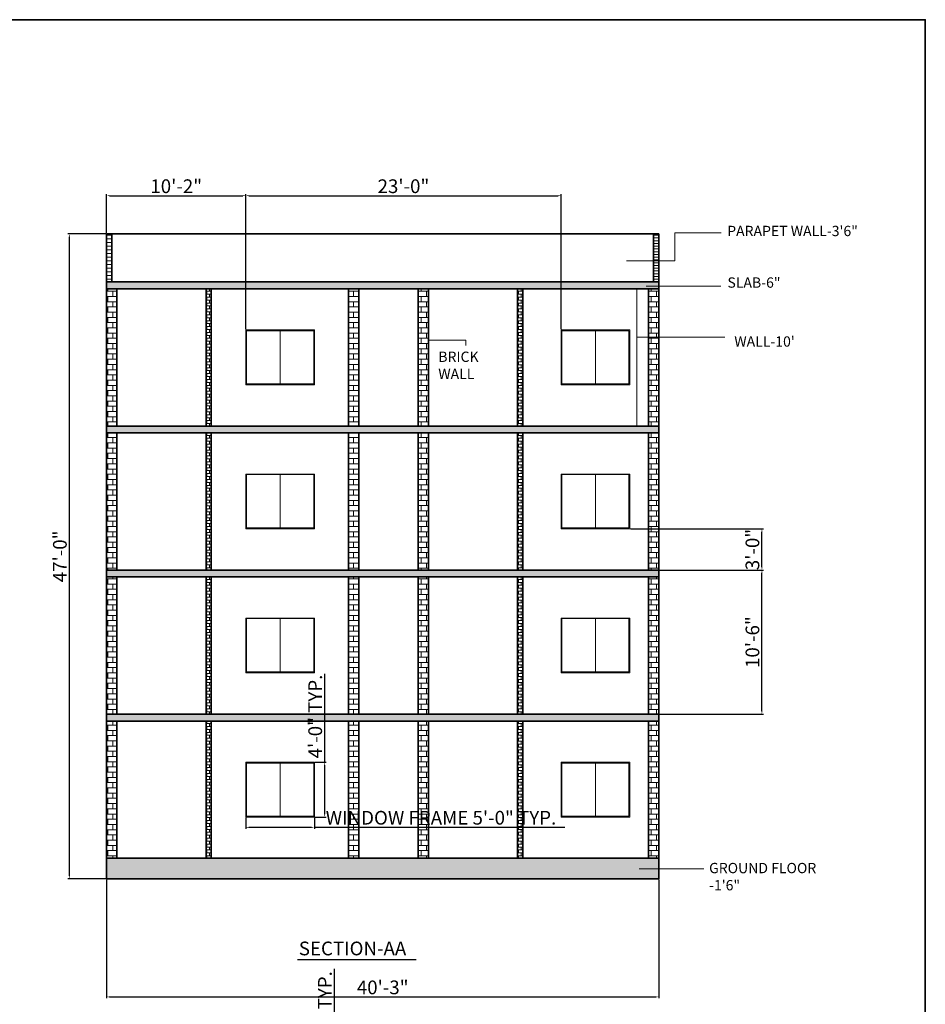
# Model space of a CAD drawing. Units: inches. Extents: x 1266 to 2869, y -408 to 3241.
# Tile 11 of 11: x 2076 to 2869, y 2380 to 3241. Entities that reach past the tile are written whole.
import ezdxf

# ---------------------------------------------------------------- set-up
doc = ezdxf.new("R2010")
doc.units = ezdxf.units.IN
for name, color, linetype, lineweight in [('A-ANNO-DIMS', 2, 'Continuous', 18), ('A-ANNO-TEXT', 7, 'Continuous', 18), ('A-ANNO-TITL', 7, 'Continuous', 25), ('A-ANNO-TTLB', 7, 'Continuous', 35), ('A-GLAZ', 4, 'Continuous', 18), ('A-SECT', 7, 'Continuous', 35), ('A-SECT-PATT', 252, 'Continuous', 13), ('A-SECT-PATT-CONC', 8, 'Continuous', 13), ('A-SECT-PATT-MASN', 8, 'Continuous', 13)]:
    doc.layers.add(name, color=color, linetype=linetype, lineweight=lineweight)
doc.styles.get("Standard").update_dxf_attribs({"font": 'arial.ttf'})
doc.dimstyles.new('ISO-25', dxfattribs={"dimtxt": 12, "dimasz": 2.5, "dimexe": 1.25, "dimexo": 0.625, "dimtad": 1, "dimdec": 0, "dimlunit": 3, "dimtxsty": 'Standard', "dimcen": 2.5, "dimadec": 0, "dimazin": 0, "dimtfac": 1, "dimtdec": 0, "dimtmove": 0, "dimatfit": 3, "dimfxl": 1, "dimarcsym": 0})

# ---------------------------------------------------------------- blocks, each defined once
blk = doc.blocks.new('WIN-SECTION-FRAME-60X48')
for p, q in [((0, 48), (0, 0)), ((0, 48), (60, 48)), ((60, 48), (60, 0)), ((0, 0), (60, 0))]:
    blk.add_line(p, q)
blk = doc.blocks.new('*D39')
at = {"layer": 'A-ANNO-DIMS', "color": 0, "lineweight": -2, "transparency": 16777216}
for p, q in [((2351.77, 2267.74), (2351.77, 2411.2)), ((2339.28, 2267.74), (2353.02, 2267.74)), ((2351.77, 2182.78), (2351.77, 2265.24)), ((2339.28, 2180.28), (2353.02, 2180.28))]:
    blk.add_line(p, q, dxfattribs=at)
at = {"layer": 'A-ANNO-DIMS', "color": 0, "transparency": 16777216}
for points in [[(2351.36, 2265.24), (2352.19, 2265.24), (2351.77, 2267.74)], [(2351.36, 2182.78), (2352.19, 2182.78), (2351.77, 2180.28)]]:
    blk.add_solid(points, dxfattribs=at)
at = {"layer": 'Defpoints', "color": 0, "transparency": 16777216}
for p in [(2338.65, 2267.74), (2351.77, 2267.74), (2338.65, 2180.28)]:
    blk.add_point(p, dxfattribs=at)
at = {"layer": 'A-ANNO-DIMS', "color": 0, "transparency": 16777216, "insert": (2344.94, 2340.72), "char_height": 12, "attachment_point": 5, "rotation": 90}
blk.add_mtext('BED 7\'-3 1/2" TYP.', dxfattribs=at)
blk = doc.blocks.new('*D51')
at = {"layer": 'A-ANNO-DIMS', "color": 0, "lineweight": -2, "transparency": 16777216}
for p, q in [((2274.21, 2543.33), (2274.21, 2533.71)), ((2334.21, 2543.33), (2334.21, 2533.71)), ((2276.71, 2534.96), (2331.71, 2534.96)), ((2334.21, 2534.96), (2553.14, 2534.96))]:
    blk.add_line(p, q, dxfattribs=at)
at = {"layer": 'A-ANNO-DIMS', "color": 0, "transparency": 16777216}
for points in [[(2276.71, 2535.38), (2276.71, 2534.54), (2274.21, 2534.96)], [(2331.71, 2535.38), (2331.71, 2534.54), (2334.21, 2534.96)]]:
    blk.add_solid(points, dxfattribs=at)
at = {"layer": 'Defpoints', "color": 0, "transparency": 16777216}
for p in [(2274.21, 2543.96), (2334.21, 2543.96), (2334.21, 2534.96)]:
    blk.add_point(p, dxfattribs=at)
at = {"layer": 'A-ANNO-DIMS', "color": 0, "transparency": 16777216, "insert": (2444.92, 2541.79), "char_height": 12, "attachment_point": 5}
blk.add_mtext('WINDOW FRAME 5\'-0" TYP.', dxfattribs=at)
blk = doc.blocks.new('*D52')
at = {"layer": 'A-ANNO-DIMS', "color": 0, "lineweight": -2, "transparency": 16777216}
for p, q in [((2343.21, 2591.96), (2343.21, 2669.34)), ((2334.83, 2591.96), (2344.46, 2591.96)), ((2343.21, 2546.46), (2343.21, 2589.46)), ((2334.83, 2543.96), (2344.46, 2543.96))]:
    blk.add_line(p, q, dxfattribs=at)
at = {"layer": 'A-ANNO-DIMS', "color": 0, "transparency": 16777216}
for points in [[(2342.79, 2589.46), (2343.63, 2589.46), (2343.21, 2591.96)], [(2342.79, 2546.46), (2343.63, 2546.46), (2343.21, 2543.96)]]:
    blk.add_solid(points, dxfattribs=at)
at = {"layer": 'Defpoints', "color": 0, "transparency": 16777216}
for p in [(2334.21, 2591.96), (2343.21, 2591.96), (2334.21, 2543.96)]:
    blk.add_point(p, dxfattribs=at)
at = {"layer": 'A-ANNO-DIMS', "color": 0, "transparency": 16777216, "insert": (2336.46, 2631.9), "char_height": 12, "attachment_point": 5, "rotation": 90}
blk.add_mtext('4\'-0" TYP.', dxfattribs=at)
blk = doc.blocks.new('*D96')
at = {"layer": 'A-ANNO-DIMS', "color": 0, "lineweight": -2, "transparency": 16777216}
for p, q in [((2152.45, 2489.33), (2152.45, 2385.4)), ((2635.45, 2489.33), (2635.45, 2385.4)), ((2154.95, 2386.65), (2632.95, 2386.65))]:
    blk.add_line(p, q, dxfattribs=at)
at = {"layer": 'A-ANNO-DIMS', "color": 0, "transparency": 16777216}
for points in [[(2154.95, 2387.07), (2154.95, 2386.23), (2152.45, 2386.65)], [(2632.95, 2387.07), (2632.95, 2386.23), (2635.45, 2386.65)]]:
    blk.add_solid(points, dxfattribs=at)
at = {"layer": 'Defpoints', "color": 0, "transparency": 16777216}
for p in [(2152.45, 2489.96), (2635.45, 2489.96), (2635.45, 2386.65)]:
    blk.add_point(p, dxfattribs=at)
at = {"layer": 'A-ANNO-DIMS', "color": 0, "transparency": 16777216, "insert": (2393.95, 2393.41), "char_height": 12, "attachment_point": 5}
blk.add_mtext('40\'-3"', dxfattribs=at)
blk = doc.blocks.new('*D97')
at = {"layer": 'A-ANNO-DIMS', "color": 0, "lineweight": -2, "transparency": 16777216}
for p, q in [((2151.83, 3053.96), (2118.6, 3053.96)), ((2119.85, 2492.46), (2119.85, 3051.46)), ((2151.83, 2489.96), (2118.6, 2489.96))]:
    blk.add_line(p, q, dxfattribs=at)
at = {"layer": 'A-ANNO-DIMS', "color": 0, "transparency": 16777216}
for points in [[(2119.43, 3051.46), (2120.27, 3051.46), (2119.85, 3053.96)], [(2119.43, 2492.46), (2120.27, 2492.46), (2119.85, 2489.96)]]:
    blk.add_solid(points, dxfattribs=at)
at = {"layer": 'Defpoints', "color": 0, "transparency": 16777216}
for p in [(2119.85, 3053.96), (2152.45, 3053.96), (2152.45, 2489.96)]:
    blk.add_point(p, dxfattribs=at)
at = {"layer": 'A-ANNO-DIMS', "color": 0, "transparency": 16777216, "insert": (2113.1, 2771.96), "char_height": 12, "attachment_point": 5, "rotation": 90}
blk.add_mtext('47\'-0"', dxfattribs=at)
blk = doc.blocks.new('*D98')
at = {"layer": 'A-ANNO-DIMS', "color": 0, "lineweight": -2, "transparency": 16777216}
for p, q in [((2636.08, 2759.96), (2726.95, 2759.96)), ((2725.7, 2636.46), (2725.7, 2757.46)), ((2636.08, 2633.96), (2726.95, 2633.96))]:
    blk.add_line(p, q, dxfattribs=at)
at = {"layer": 'A-ANNO-DIMS', "color": 0, "transparency": 16777216}
for points in [[(2725.28, 2757.46), (2726.12, 2757.46), (2725.7, 2759.96)], [(2725.28, 2636.46), (2726.12, 2636.46), (2725.7, 2633.96)]]:
    blk.add_solid(points, dxfattribs=at)
at = {"layer": 'Defpoints', "color": 0, "transparency": 16777216}
for p in [(2635.45, 2759.96), (2725.7, 2759.96), (2635.45, 2633.96)]:
    blk.add_point(p, dxfattribs=at)
at = {"layer": 'A-ANNO-DIMS', "color": 0, "transparency": 16777216, "insert": (2718.95, 2696.96), "char_height": 12, "attachment_point": 5, "rotation": 90}
blk.add_mtext('10\'-6"', dxfattribs=at)
blk = doc.blocks.new('*D99')
at = {"layer": 'A-ANNO-DIMS', "color": 0, "lineweight": -2, "transparency": 16777216}
for p, q in [((2152.45, 3054.58), (2152.45, 3088.64)), ((2154.95, 3087.39), (2271.71, 3087.39)), ((2274.21, 2970.58), (2274.21, 3088.64))]:
    blk.add_line(p, q, dxfattribs=at)
at = {"layer": 'A-ANNO-DIMS', "color": 0, "transparency": 16777216}
for points in [[(2154.95, 3087.8), (2154.95, 3086.97), (2152.45, 3087.39)], [(2271.71, 3087.8), (2271.71, 3086.97), (2274.21, 3087.39)]]:
    blk.add_solid(points, dxfattribs=at)
at = {"layer": 'Defpoints', "color": 0, "transparency": 16777216}
for p in [(2274.21, 3087.39), (2152.45, 3053.96), (2274.21, 2969.96)]:
    blk.add_point(p, dxfattribs=at)
at = {"layer": 'A-ANNO-DIMS', "color": 0, "transparency": 16777216, "insert": (2213.33, 3094.14), "char_height": 12, "attachment_point": 5}
blk.add_mtext('10\'-2"', dxfattribs=at)
blk = doc.blocks.new('*D100')
at = {"layer": 'A-ANNO-DIMS', "color": 0, "lineweight": -2, "transparency": 16777216}
for p, q in [((2274.21, 2970.58), (2274.21, 3088.64)), ((2276.71, 3087.39), (2547.51, 3087.39)), ((2550.01, 2970.58), (2550.01, 3088.64))]:
    blk.add_line(p, q, dxfattribs=at)
at = {"layer": 'A-ANNO-DIMS', "color": 0, "transparency": 16777216}
for points in [[(2276.71, 3087.8), (2276.71, 3086.97), (2274.21, 3087.39)], [(2547.51, 3087.8), (2547.51, 3086.97), (2550.01, 3087.39)]]:
    blk.add_solid(points, dxfattribs=at)
at = {"layer": 'Defpoints', "color": 0, "transparency": 16777216}
for p in [(2550.01, 3087.39), (2274.21, 2969.96), (2550.01, 2969.96)]:
    blk.add_point(p, dxfattribs=at)
at = {"layer": 'A-ANNO-DIMS', "color": 0, "transparency": 16777216, "insert": (2412.11, 3094.14), "char_height": 12, "attachment_point": 5}
blk.add_mtext('23\'-0"', dxfattribs=at)
blk = doc.blocks.new('*D101')
at = {"layer": 'A-ANNO-DIMS', "color": 0, "lineweight": -2, "transparency": 16777216}
for p, q in [((2610.64, 2795.96), (2726.95, 2795.96)), ((2725.7, 2762.46), (2725.7, 2793.46)), ((2636.08, 2759.96), (2726.95, 2759.96))]:
    blk.add_line(p, q, dxfattribs=at)
at = {"layer": 'A-ANNO-DIMS', "color": 0, "transparency": 16777216}
for points in [[(2725.28, 2793.46), (2726.12, 2793.46), (2725.7, 2795.96)], [(2725.28, 2762.46), (2726.12, 2762.46), (2725.7, 2759.96)]]:
    blk.add_solid(points, dxfattribs=at)
at = {"layer": 'Defpoints', "color": 0, "transparency": 16777216}
for p in [(2610.01, 2795.96), (2725.7, 2795.96), (2635.45, 2759.96)]:
    blk.add_point(p, dxfattribs=at)
at = {"layer": 'A-ANNO-DIMS', "color": 0, "transparency": 16777216, "insert": (2718.94, 2777.96), "char_height": 12, "attachment_point": 5, "rotation": 90}
blk.add_mtext('3\'-0"', dxfattribs=at)

msp = doc.modelspace()

# ---------------------------------------------------------------- hatches: boundary and pattern name
at = {"layer": 'A-SECT-PATT', "transparency": 33554536}
h = msp.add_hatch(color=256, dxfattribs=at)
h.dxf.hatch_style = 1
h.paths.add_polyline_path([(2635.45, 3011.96), (2152.45, 3011.96), (2152.45, 3005.96), (2635.45, 3005.96)])
h.paths.add_polyline_path([(2635.45, 2885.96), (2152.45, 2885.96), (2152.45, 2879.96), (2635.45, 2879.96)])
h.paths.add_polyline_path([(2635.45, 2759.96), (2152.45, 2759.96), (2152.45, 2753.96), (2635.45, 2753.96)])
h.paths.add_polyline_path([(2635.45, 2633.96), (2152.45, 2633.96), (2152.45, 2627.96), (2635.45, 2627.96)])
at = {"layer": 'A-SECT-PATT-CONC'}
h = msp.add_hatch(dxfattribs=at)
h.set_pattern_fill('AR-CONC', color=256, scale=0.107, style=0)
h.paths.add_polyline_path([(2152.45, 2489.96), (2635.45, 2489.96), (2635.45, 2507.96), (2152.45, 2507.96)])
at = {"layer": 'A-SECT-PATT-MASN'}
h = msp.add_hatch(dxfattribs=at)
h.set_pattern_fill('LINE', color=256, scale=1.007874, style=0)
h.paths.add_polyline_path([(2152.45, 3011.96), (2157.08, 3011.96), (2157.08, 3053.96), (2152.45, 3053.96)])
h = msp.add_hatch(dxfattribs=at)
h.set_pattern_fill('LINE', color=256, scale=0.7559055, style=0)
h.paths.add_polyline_path([(2630.96, 3011.96), (2635.45, 3011.96), (2635.45, 3053.96), (2630.96, 3053.96)])
h = msp.add_hatch(dxfattribs=at)
h.set_pattern_fill('BRICK', color=256, scale=0.72, style=0)
h.paths.add_polyline_path([(2152.45, 2885.96), (2161.45, 2885.96), (2161.45, 3005.96), (2152.45, 3005.96)])
h = msp.add_hatch(dxfattribs=at)
h.set_pattern_fill('BRICK', color=256, scale=0.405, style=0)
h.paths.add_polyline_path([(2239.45, 2885.96), (2243.95, 2885.96), (2243.95, 3005.96), (2239.45, 3005.96)])
h = msp.add_hatch(dxfattribs=at)
h.set_pattern_fill('BRICK', color=256, scale=0.72, style=0)
h.paths.add_polyline_path([(2363.95, 2885.96), (2372.95, 2885.96), (2372.95, 3005.96), (2363.95, 3005.96)])
h = msp.add_hatch(dxfattribs=at)
h.set_pattern_fill('BRICK', color=256, scale=0.72, style=0)
h.paths.add_polyline_path([(2424.95, 2885.96), (2433.95, 2885.96), (2433.95, 3005.96), (2424.95, 3005.96)])
h = msp.add_hatch(dxfattribs=at)
h.set_pattern_fill('BRICK', color=256, scale=0.405, style=0)
h.paths.add_polyline_path([(2511.95, 2885.96), (2516.45, 2885.96), (2516.45, 3005.96), (2511.95, 3005.96)])
h = msp.add_hatch(dxfattribs=at)
h.set_pattern_fill('BRICK', color=256, scale=0.72, style=0)
h.paths.add_polyline_path([(2626.45, 2885.96), (2635.45, 2885.96), (2635.45, 3005.96), (2626.45, 3005.96)])
h = msp.add_hatch(dxfattribs=at)
h.set_pattern_fill('BRICK', color=256, scale=0.72, style=0)
h.paths.add_polyline_path([(2152.45, 2759.96), (2161.45, 2759.96), (2161.45, 2879.96), (2152.45, 2879.96)])
h = msp.add_hatch(dxfattribs=at)
h.set_pattern_fill('BRICK', color=256, scale=0.405, style=0)
h.paths.add_polyline_path([(2239.45, 2759.96), (2243.95, 2759.96), (2243.95, 2879.96), (2239.45, 2879.96)])
h = msp.add_hatch(dxfattribs=at)
h.set_pattern_fill('BRICK', color=256, scale=0.72, style=0)
h.paths.add_polyline_path([(2363.95, 2759.96), (2372.95, 2759.96), (2372.95, 2879.96), (2363.95, 2879.96)])
h = msp.add_hatch(dxfattribs=at)
h.set_pattern_fill('BRICK', color=256, scale=0.72, style=0)
h.paths.add_polyline_path([(2424.95, 2759.96), (2433.95, 2759.96), (2433.95, 2879.96), (2424.95, 2879.96)])
h = msp.add_hatch(dxfattribs=at)
h.set_pattern_fill('BRICK', color=256, scale=0.405, style=0)
h.paths.add_polyline_path([(2511.95, 2759.96), (2516.45, 2759.96), (2516.45, 2879.96), (2511.95, 2879.96)])
h = msp.add_hatch(dxfattribs=at)
h.set_pattern_fill('BRICK', color=256, scale=0.72, style=0)
h.paths.add_polyline_path([(2626.45, 2759.96), (2635.45, 2759.96), (2635.45, 2879.96), (2626.45, 2879.96)])
h = msp.add_hatch(dxfattribs=at)
h.set_pattern_fill('BRICK', color=256, scale=0.72, style=0)
h.paths.add_polyline_path([(2152.45, 2633.96), (2161.45, 2633.96), (2161.45, 2753.96), (2152.45, 2753.96)])
h = msp.add_hatch(dxfattribs=at)
h.set_pattern_fill('BRICK', color=256, scale=0.405, style=0)
h.paths.add_polyline_path([(2239.45, 2633.96), (2243.95, 2633.96), (2243.95, 2753.96), (2239.45, 2753.96)])
h = msp.add_hatch(dxfattribs=at)
h.set_pattern_fill('BRICK', color=256, scale=0.72, style=0)
h.paths.add_polyline_path([(2363.95, 2633.96), (2372.95, 2633.96), (2372.95, 2753.96), (2363.95, 2753.96)])
h = msp.add_hatch(dxfattribs=at)
h.set_pattern_fill('BRICK', color=256, scale=0.72, style=0)
h.paths.add_polyline_path([(2424.95, 2633.96), (2433.95, 2633.96), (2433.95, 2753.96), (2424.95, 2753.96)])
h = msp.add_hatch(dxfattribs=at)
h.set_pattern_fill('BRICK', color=256, scale=0.405, style=0)
h.paths.add_polyline_path([(2511.95, 2633.96), (2516.45, 2633.96), (2516.45, 2753.96), (2511.95, 2753.96)])
h = msp.add_hatch(dxfattribs=at)
h.set_pattern_fill('BRICK', color=256, scale=0.72, style=0)
h.paths.add_polyline_path([(2626.45, 2633.96), (2635.45, 2633.96), (2635.45, 2753.96), (2626.45, 2753.96)])
h = msp.add_hatch(dxfattribs=at)
h.set_pattern_fill('BRICK', color=256, scale=0.72, style=0)
h.paths.add_polyline_path([(2152.45, 2507.96), (2161.45, 2507.96), (2161.45, 2627.96), (2152.45, 2627.96)])
h = msp.add_hatch(dxfattribs=at)
h.set_pattern_fill('BRICK', color=256, scale=0.405, style=0)
h.paths.add_polyline_path([(2239.45, 2507.96), (2243.95, 2507.96), (2243.95, 2627.96), (2239.45, 2627.96)])
h = msp.add_hatch(dxfattribs=at)
h.set_pattern_fill('BRICK', color=256, scale=0.72, style=0)
h.paths.add_polyline_path([(2363.95, 2507.96), (2372.95, 2507.96), (2372.95, 2627.96), (2363.95, 2627.96)])
h = msp.add_hatch(dxfattribs=at)
h.set_pattern_fill('BRICK', color=256, scale=0.72, style=0)
h.paths.add_polyline_path([(2424.95, 2507.96), (2433.95, 2507.96), (2433.95, 2627.96), (2424.95, 2627.96)])
h = msp.add_hatch(dxfattribs=at)
h.set_pattern_fill('BRICK', color=256, scale=0.405, style=0)
h.paths.add_polyline_path([(2511.95, 2507.96), (2516.45, 2507.96), (2516.45, 2627.96), (2511.95, 2627.96)])
h = msp.add_hatch(dxfattribs=at)
h.set_pattern_fill('BRICK', color=256, scale=0.72, style=0)
h.paths.add_polyline_path([(2626.45, 2507.96), (2635.45, 2507.96), (2635.45, 2627.96), (2626.45, 2627.96)])

# ---------------------------------------------------------------- linework, layer by layer
at = {"layer": 'A-ANNO-TEXT'}
for p, q in [((2690.17, 3054.79), (2649.45, 3054.79)), ((2649.45, 3054.79), (2649.45, 3030.52)), ((2649.45, 3030.52), (2607.26, 3030.52)), ((2616.31, 2963.78), (2616.31, 3005.96)), ((2616.31, 3005.96), (2616.31, 2885.96)), ((2624.47, 3008.37), (2689.62, 3008.37)), ((2616.31, 2963.78), (2693.1, 2963.78)), ((2433.95, 2961.09), (2466.79, 2961.09)), ((2466.79, 2961.09), (2466.79, 2956.26)), ((2618.31, 2498.6), (2674.88, 2498.6))]:
    msp.add_line(p, q, dxfattribs=at)
at = {"layer": 'A-ANNO-TITL'}
msp.add_line((2319.44, 2419.25), (2423.24, 2419.25), dxfattribs=at)
at = {"layer": 'A-ANNO-TTLB'}
msp.add_lwpolyline([(1266.23, 3241.34), (2868.62, 3241.34), (2868.62, 986.84), (1266.23, 986.84)], close=True, dxfattribs=at)
at = {"layer": 'A-GLAZ'}
for p, q in [((2304.24, 2969.24), (2304.24, 2922.73)), ((2580.01, 2969.24), (2580.01, 2922.73)), ((2304.24, 2843.55), (2304.24, 2797.04)), ((2580.01, 2843.96), (2580.01, 2797.04)), ((2304.24, 2717.53), (2304.24, 2671.02)), ((2580.01, 2717.53), (2580.01, 2671.02)), ((2304.24, 2591.15), (2304.24, 2544.64)), ((2580.01, 2591.15), (2580.01, 2544.64))]:
    msp.add_line(p, q, dxfattribs=at)
for points in [[(2274.89, 2969.24), (2333.59, 2969.24), (2333.59, 2922.73), (2274.89, 2922.73)], [(2550.66, 2969.24), (2609.36, 2969.24), (2609.36, 2922.73), (2550.66, 2922.73)], [(2274.89, 2843.55), (2333.59, 2843.55), (2333.59, 2797.04), (2274.89, 2797.04)], [(2550.66, 2843.55), (2609.36, 2843.55), (2609.36, 2797.04), (2550.66, 2797.04)], [(2274.89, 2717.53), (2333.59, 2717.53), (2333.59, 2671.02), (2274.89, 2671.02)], [(2550.66, 2717.53), (2609.36, 2717.53), (2609.36, 2671.02), (2550.66, 2671.02)], [(2274.89, 2591.15), (2333.59, 2591.15), (2333.59, 2544.64), (2274.89, 2544.64)], [(2550.66, 2591.15), (2609.36, 2591.15), (2609.36, 2544.64), (2550.66, 2544.64)]]:
    msp.add_lwpolyline(points, close=True, dxfattribs=at)
at = {"layer": 'A-SECT'}
for p, q in [((2152.45, 3053.96), (2635.45, 3053.96)), ((2152.45, 2867.96), (2152.45, 3053.96)), ((2157.08, 3011.96), (2157.08, 3053.96)), ((2630.96, 3011.96), (2630.96, 3053.96)), ((2635.45, 2867.96), (2635.45, 3053.96)), ((2152.45, 3011.96), (2635.45, 3011.96)), ((2152.45, 3005.96), (2635.45, 3005.96)), ((2161.45, 3005.96), (2161.45, 2885.96)), ((2239.45, 3005.96), (2239.45, 2885.96)), ((2243.95, 3005.96), (2243.95, 2885.96)), ((2363.95, 3005.96), (2363.95, 2885.96)), ((2372.95, 3005.96), (2372.95, 2885.96)), ((2424.95, 3005.96), (2424.95, 2885.96)), ((2433.95, 3005.96), (2433.95, 2885.96)), ((2511.95, 3005.96), (2511.95, 2885.96)), ((2516.45, 3005.96), (2516.45, 2885.96)), ((2626.45, 3005.96), (2626.45, 2885.96)), ((2152.45, 2741.96), (2152.45, 2927.96)), ((2635.45, 2741.96), (2635.45, 2927.96)), ((2152.45, 2885.96), (2635.45, 2885.96)), ((2152.45, 2879.96), (2635.45, 2879.96)), ((2161.45, 2879.96), (2161.45, 2759.96)), ((2239.45, 2879.96), (2239.45, 2759.96)), ((2243.95, 2879.96), (2243.95, 2759.96)), ((2363.95, 2879.96), (2363.95, 2759.96)), ((2372.95, 2879.96), (2372.95, 2759.96)), ((2424.95, 2879.96), (2424.95, 2759.96)), ((2433.95, 2879.96), (2433.95, 2759.96)), ((2511.95, 2879.96), (2511.95, 2759.96)), ((2516.45, 2879.96), (2516.45, 2759.96)), ((2626.45, 2879.96), (2626.45, 2759.96)), ((2152.45, 2615.96), (2152.45, 2801.96)), ((2635.45, 2615.96), (2635.45, 2801.96)), ((2152.45, 2759.96), (2635.45, 2759.96)), ((2152.45, 2753.96), (2635.45, 2753.96)), ((2161.45, 2753.96), (2161.45, 2633.96)), ((2239.45, 2753.96), (2239.45, 2633.96)), ((2243.95, 2753.96), (2243.95, 2633.96)), ((2363.95, 2753.96), (2363.95, 2633.96)), ((2372.95, 2753.96), (2372.95, 2633.96)), ((2424.95, 2753.96), (2424.95, 2633.96)), ((2433.95, 2753.96), (2433.95, 2633.96)), ((2511.95, 2753.96), (2511.95, 2633.96)), ((2516.45, 2753.96), (2516.45, 2633.96)), ((2626.45, 2753.96), (2626.45, 2633.96)), ((2152.45, 2489.96), (2152.45, 2675.96)), ((2635.45, 2489.96), (2635.45, 2675.96)), ((2152.45, 2633.96), (2635.45, 2633.96)), ((2152.45, 2627.96), (2635.45, 2627.96)), ((2161.45, 2627.96), (2161.45, 2507.96)), ((2239.45, 2627.96), (2239.45, 2507.96)), ((2243.95, 2627.96), (2243.95, 2507.96)), ((2363.95, 2627.96), (2363.95, 2507.96)), ((2372.95, 2627.96), (2372.95, 2507.96)), ((2424.95, 2627.96), (2424.95, 2507.96)), ((2433.95, 2627.96), (2433.95, 2507.96)), ((2511.95, 2627.96), (2511.95, 2507.96)), ((2516.45, 2627.96), (2516.45, 2507.96)), ((2626.45, 2627.96), (2626.45, 2507.96)), ((2152.45, 2507.96), (2635.45, 2507.96)), ((2152.45, 2489.96), (2635.45, 2489.96))]:
    msp.add_line(p, q, dxfattribs=at)

# ---------------------------------------------------------------- block references
at = {"layer": 'A-GLAZ'}
for p in [(2274.21, 2921.96), (2550.01, 2921.96), (2274.21, 2795.96), (2550.01, 2795.96), (2274.21, 2669.96), (2550.01, 2669.96), (2274.21, 2543.96), (2550.01, 2543.96)]:
    msp.add_blockref('WIN-SECTION-FRAME-60X48', p, dxfattribs=at)

# ---------------------------------------------------------------- texts
at = {"layer": 'A-ANNO-TEXT', "char_height": 9, "attachment_point": 1}
for s, width, insert in [('PARAPET WALL-3\'6"', 120.1516, (2695.32, 3061.06)), ('SLAB-6"', 63.5654, (2695.53, 3015.93)), ("WALL-10'", 97.0657, (2701.54, 2964.39)), ('BRICK WALL', 31.9297, (2442.59, 2951.01)), ('GROUND FLOOR -1\'6"', 122.7321, (2679.48, 2503.85))]:
    msp.add_mtext_dynamic_manual_height_columns(s, width=width, gutter_width=12.5, heights=[0], dxfattribs=dict(at, insert=insert))
at = {"layer": 'A-ANNO-TITL', "insert": (2320.56, 2435.02), "char_height": 12, "attachment_point": 1}
msp.add_mtext_dynamic_manual_height_columns('SECTION-AA', width=217.5226, gutter_width=12.5, heights=[0], dxfattribs=at)

# ---------------------------------------------------------------- dimensions: what is measured, and where the dimension line sits
at = {"layer": 'A-ANNO-DIMS'}
for base, p1, p2, picture, middle in [((2274.21, 3087.39), (2152.45, 3053.96), (2274.21, 2969.96), '*D99', (2213.33, 3094.14)), ((2550.01, 3087.39), (2274.21, 2969.96), (2550.01, 2969.96), '*D100', (2412.11, 3094.14)), ((2635.45, 2386.65), (2152.45, 2489.96), (2635.45, 2489.96), '*D96', (2393.95, 2393.41))]:
    dim = msp.add_linear_dim(base=base, p1=p1, p2=p2, dimstyle='ISO-25', override={"dimdec": 1, "dimlfac": 1, "dimrnd": 0, "dimzin": 1, "dimdsep": 46, "dimlunit": 4, "dimfrac": 2}, dxfattribs=at)
    dim.commit()
    dim.dimension.update_dxf_attribs({"geometry": picture, "text_midpoint": middle})
for base, p1, p2, picture, middle in [((2119.85, 3053.96), (2152.45, 2489.96), (2152.45, 3053.96), '*D97', (2113.1, 2771.96)), ((2725.7, 2795.96), (2635.45, 2759.96), (2610.01, 2795.96), '*D101', (2718.94, 2777.96)), ((2725.7, 2759.96), (2635.45, 2633.96), (2635.45, 2759.96), '*D98', (2718.95, 2696.96))]:
    dim = msp.add_linear_dim(base=base, p1=p1, p2=p2, angle=90, dimstyle='ISO-25', override={"dimdec": 1, "dimlfac": 1, "dimrnd": 0, "dimzin": 1, "dimdsep": 46, "dimlunit": 4, "dimfrac": 2}, dxfattribs=at)
    dim.commit()
    dim.dimension.update_dxf_attribs({"geometry": picture, "text_midpoint": middle})
for base, p1, p2, text, picture, middle in [((2343.21, 2591.96), (2334.21, 2543.96), (2334.21, 2591.96), '<> TYP.', '*D52', (2336.46, 2631.9)), ((2351.77, 2267.74), (2338.65, 2180.28), (2338.65, 2267.74), 'BED <> TYP.', '*D39', (2344.94, 2340.72))]:
    dim = msp.add_linear_dim(base=base, p1=p1, p2=p2, angle=90, text=text, dimstyle='ISO-25', override={"dimdec": 1, "dimlfac": 1, "dimrnd": 0, "dimzin": 1, "dimdsep": 46, "dimlunit": 4, "dimfrac": 2}, dxfattribs=at)
    dim.commit()
    dim.dimension.update_dxf_attribs({"geometry": picture, "text_midpoint": middle})
dim = msp.add_linear_dim(base=(2334.21, 2534.96), p1=(2274.21, 2543.96), p2=(2334.21, 2543.96), text='WINDOW FRAME <> TYP.', dimstyle='ISO-25', override={"dimdec": 1, "dimlfac": 1, "dimrnd": 0, "dimzin": 1, "dimdsep": 46, "dimlunit": 4, "dimfrac": 2}, dxfattribs=at)
dim.commit()
dim.dimension.update_dxf_attribs({"geometry": '*D51', "text_midpoint": (2444.92, 2541.79)})

doc.saveas('drawing.dxf')
